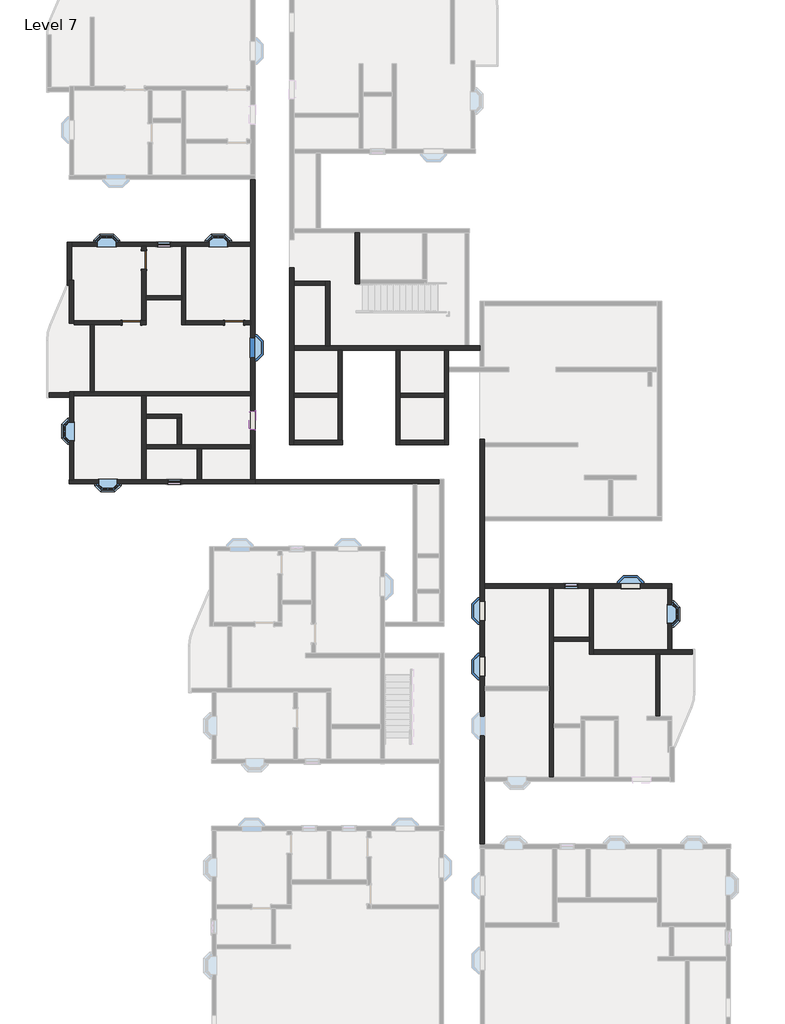
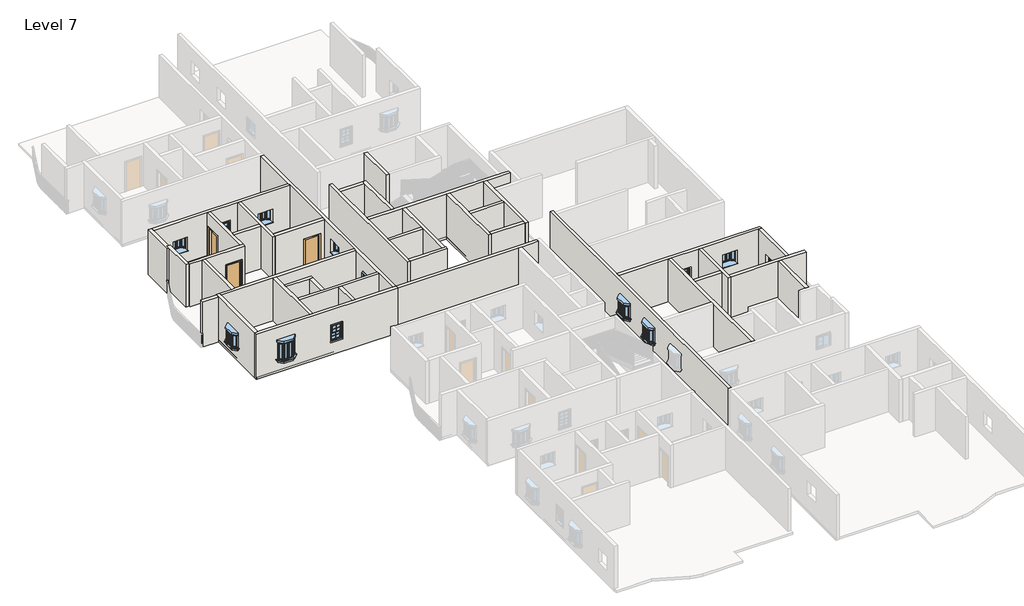
# One storey, part 3 of 14: 40 walls, 13 windows, 3 doors.
# Revit data of these elements (continued)
# Element 24 (IfcWall, "9\"") (continued)
#   Materials on its faces: "Default Wall", "Cherry"
# Element 25 (IfcWall, "9\"")
#   Top Offset = 0' - 0"
#   Base Offset = 0' - 0"
#   wall height = 10' - 0"
#   Phase Created = New Construction
#   Base Constraint = Level 7
#   Top Constraint = Level 8
#   Materials on its faces: "Default Wall", "Parking Stripe"
# Element 26 (IfcWall, "9\"")
#   Top Offset = 0' - 0"
#   Base Offset = 0' - 0"
#   wall height = 10' - 0"
#   Phase Created = New Construction
#   Base Constraint = Level 7
#   Top Constraint = Level 8
#   Materials on its faces: "Default Wall", "Earth", "Cherry"
# Element 27 (IfcWall, "9\"")
#   Top Offset = 0' - 0"
#   Base Offset = 0' - 0"
#   wall height = 10' - 0"
#   Phase Created = New Construction
#   Base Constraint = Level 7
#   Top Constraint = Level 8
#   Materials on its faces: "Default Wall", "Default Mass Interior Wall"
# Element 28 (IfcWall, "9\"")
#   Top Offset = 0' - 0"
#   Base Offset = 0' - 0"
#   wall height = 10' - 0"
#   Phase Created = New Construction
#   Base Constraint = Level 7
#   Top Constraint = Level 8
#   Materials on its faces: "Default Wall"
# Element 29 (IfcWall, "9\"")
#   Top Offset = 0' - 0"
#   Base Offset = 0' - 0"
#   wall height = 10' - 0"
#   Phase Created = New Construction
#   Base Constraint = Level 7
#   Top Constraint = Level 8
#   Materials on its faces: "Default Wall", "Default Mass Interior Wall", "Earth"
# Elements 30, 33, 34, 35, 36, 37, 38, 39, 40, 41 (IfcWall, "9\" w")
#   Top Offset = 0' - 0"
#   Base Offset = 0' - 0"
#   wall height = 10' - 0"
#   Phase Created = New Construction
#   Base Constraint = Level 7
#   Top Constraint = Level 8
#   Materials on its faces: "Default Wall"
# Element 31 (IfcWall, "9\" w")
#   Top Offset = 0' - 0"
#   Base Offset = 0' - 0"
#   wall height = 10' - 0"
#   Phase Created = New Construction
#   Base Constraint = Level 7
#   Top Constraint = Level 8
#   Materials on its faces: "Default Wall", "Earth"
# Element 32 (IfcWall, "9\" w")
#   Top Offset = 0' - 0"
#   Base Offset = 0' - 0"
#   wall height = 10' - 0"
#   Phase Created = New Construction
#   Base Constraint = Level 7
#   Top Constraint = Level 8
#   Materials on its faces: "Default Wall", "Brick, Soldier Course"
# Element 42 (IfcWall, "9\" w")
#   Top Offset = 0' - 0"
#   Base Offset = 0' - 0"
#   wall height = 10' - 0"
#   Phase Created = New Construction
#   Base Constraint = Level 7
#   Top Constraint = Level 8
#   Materials on its faces: "Default Wall", "Wood - Stained"
# Element 43 (IfcWall, "9\" w")
#   Top Offset = 0' - 0"
#   Base Offset = 0' - 0"
#   wall height = 10' - 0"
#   Phase Created = New Construction
#   Base Constraint = Level 7
#   Top Constraint = Level 8
#   Materials on its faces: "Default Wall", "Acoustic Ceiling Tile 24 x 24"
# Element 44 (IfcWindow, "910x1210mm")
#   Mark = "416"
#   Phase Created = New Construction
#   Materials on its faces: "Window Frame", "Glass"
# Element 45 (IfcWindow, "910x910mm")
#   Mark = "392"
#   Phase Created = New Construction
#   Materials on its faces: "Window Frame", "Glass"
# Element 46 (IfcWindow, "910x910mm")
#   Mark = "393"
#   Phase Created = New Construction
#   Materials on its faces: "Window Frame", "Glass"
# Element 47 (IfcWindow, "910x910mm")
#   Mark = "365"
#   Phase Created = New Construction
#   Materials on its faces: "Window Frame", "Glass"
# Element 48 (IfcWindow, "910x910mm")
#   Mark = "366"
#   Phase Created = New Construction
#   Materials on its faces: "Window Frame", "Glass"
# Element 49 (IfcWindow, "910x910mm")
#   Mark = "367"
#   Phase Created = New Construction
#   Materials on its faces: "Window Frame", "Glass"
# Element 50 (IfcWindow, "910x910mm")
#   Mark = "368"
#   Phase Created = New Construction
#   Materials on its faces: "Window Frame", "Glass"
# Element 51 (IfcWindow, "910x910mm")
#   Mark = "390"
#   Phase Created = New Construction
#   Materials on its faces: "Window Frame", "Glass"
# Element 52 (IfcWindow, "910x910mm")
#   Mark = "391"
#   Phase Created = New Construction
#   Materials on its faces: "Window Frame", "Glass"
# Element 53 (IfcWindow, "Window-Double-Hung : 26\" x 42\"")
#   Mark = "414"
#   Window Inset = 0' - 0"
#   Interior Wall Closure = 0' - 1 1/2"
#   Frame Extension = 0' - 1 1/4"
#   Exterior Wall Closure = 0' - 0 1/2"
#   Interior Trim Visibility = yes
#   Indicator Visibility = yes
#   Exterior Trim Visibility = yes
#   Phase Created = New Construction
#   Materials on its faces: "Wood - Stained", "Glass", "Clad - White"
# Element 54 (IfcWindow, "Window-Double-Hung : 26\" x 42\"")
#   Mark = "403"
#   Window Inset = 0' - 0"
#   Interior Wall Closure = 0' - 1 1/2"
#   Frame Extension = 0' - 1 1/4"
#   Exterior Wall Closure = 0' - 0 1/2"
#   Interior Trim Visibility = yes
#   Indicator Visibility = yes
#   Exterior Trim Visibility = yes
#   Phase Created = New Construction
#   Materials on its faces: "Wood - Stained", "Glass", "Clad - White"
# Element 55 (IfcWindow, "Window-Double-Hung : 26\" x 42\"")
#   Mark = "404"
#   Window Inset = 0' - 0"
#   Interior Wall Closure = 0' - 1 1/2"
#   Frame Extension = 0' - 1 1/4"
#   Exterior Wall Closure = 0' - 0 1/2"
#   Interior Trim Visibility = yes
#   Indicator Visibility = yes
#   Exterior Trim Visibility = yes
#   Phase Created = New Construction
#   Materials on its faces: "Wood - Stained", "Glass", "Clad - White"
# Element 56 (IfcWindow, "Windows_Sgl_w-Glazing_Bars : 910x910mm")
#   Mark = "399"
#   Phase Created = New Construction
#   Materials on its faces: "Window Frame", "Glass"
# Materials
#   "Door - Panel": class "Wood", colour RGB 210 159 95, transparency 0, Cost = 0
#   "Door - Frame": colour RGB 118 70 51, transparency 0, Cost = 0
#   "Window Frame": colour RGB 249 249 249, transparency 0
#   "Glass": class "Glass", colour RGB 0 128 192, transparency 0.75, Description = "Soda Lime Glass", Cost = 0
#   "Wood - Stained": class "Wood", colour RGB 224 178 126, transparency 0, Cost = 0
#   "Clad - White": class "Wood", colour RGB 242 242 238, transparency 0, Cost = 0
#   "Default Wall": colour RGB 128 128 128, transparency 0, Cost = 0
#   "Acoustic Ceiling Tile 24 x 24": class "Generic", colour RGB 232 232 232, transparency 0, Description = "Acoustic Ceiling Tile 24 x 24", Cost = 0
#   "Cherry": class "Wood", colour RGB 226 177 128, transparency 0, Description = "Prunus Serotina", Cost = 0
#   "Parking Stripe": class "Paint", colour RGB 250 250 91, transparency 0, Cost = 0
#   "Earth": class "Generic", colour RGB 97 75 62, transparency 0, Description = "Soil", Cost = 0
#   "Default Mass Interior Wall": class "Generic", colour RGB 195 229 126, transparency 0, Cost = 0
#   "Brick, Soldier Course": class "Masonry", colour RGB 170 98 104, transparency 0, Description = "Common brick soldier coursed", Cost = 0
